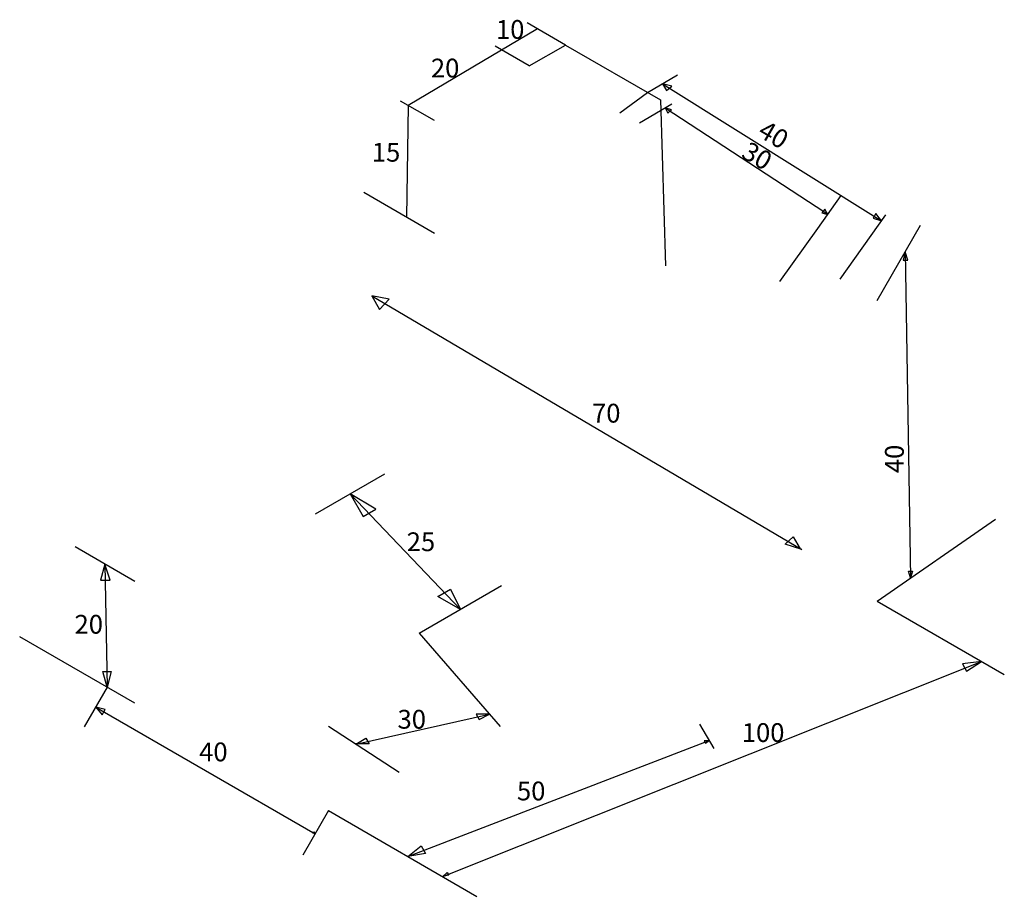
# Model space of a CAD drawing. Units: inches. Extents: x 17467 to 446717, y 8017 to 206428.
# Tile 1 of 2: x 17467 to 17598, y 8017 to 8134. Entities that reach past the tile are written whole.
import ezdxf

# ---------------------------------------------------------------- set-up
doc = ezdxf.new("R2010")
doc.units = ezdxf.units.IN
doc.layers.add('M-DIMS', color=2, linetype='Continuous', lineweight=25)
doc.layers.add('M-TEXT', color=7, linetype='Continuous', lineweight=25)
doc.styles.get("Standard").update_dxf_attribs({"font": 'arial.ttf'})

msp = doc.modelspace()

# ---------------------------------------------------------------- linework, layer by layer
at = {"layer": 'M-DIMS'}
for p, q in [((17539.99, 8130.15), (17534.91, 8133.09)), ((17536.29, 8132.29), (17519.07, 8122.12)), ((17535.19, 8127.38), (17539.99, 8130.15)), ((17539.99, 8130.15), (17552.65, 8122.84)), ((17535.19, 8127.38), (17530.64, 8130.01)), ((17550.91, 8123.85), (17554.91, 8126.16)), ((17552.91, 8125), (17582.07, 8106.74)), ((17552.91, 8125), (17553.45, 8124.08)), ((17554.14, 8124.69), (17552.91, 8125)), ((17547.26, 8121.13), (17550.91, 8123.85)), ((17553.45, 8124.08), (17554.14, 8124.69)), ((17522.57, 8120.09), (17518.07, 8122.69)), ((17549.84, 8119.79), (17554.18, 8122.3)), ((17552.65, 8122.84), (17553.33, 8100.75)), ((17519.07, 8122.12), (17518.87, 8107.23)), ((17553.26, 8121.77), (17574.5, 8107.89)), ((17553.26, 8121.77), (17553.65, 8121.09)), ((17554.12, 8121.53), (17553.26, 8121.77)), ((17553.65, 8121.09), (17554.12, 8121.53)), ((17522.57, 8105.09), (17513.16, 8110.53)), ((17573.57, 8105.75), (17576.68, 8110.11)), ((17574.5, 8108.29), (17574.11, 8107.83)), ((17574.9, 8107.6), (17574.5, 8108.29)), ((17574.5, 8107.89), (17574.9, 8107.6)), ((17574.11, 8107.83), (17574.9, 8107.6)), ((17576.57, 8098.99), (17582.64, 8107.54)), ((17581.31, 8107.72), (17580.97, 8107.12)), ((17580.97, 8107.12), (17582.07, 8106.74)), ((17582.07, 8106.74), (17581.31, 8107.72)), ((17568.52, 8098.66), (17573.57, 8105.75)), ((17581.47, 8096.15), (17587.26, 8106.17)), ((17585.21, 8102.63), (17584.94, 8101.54)), ((17585.21, 8102.63), (17585.94, 8059.25)), ((17585.57, 8101.54), (17585.21, 8102.63)), ((17584.94, 8101.54), (17585.57, 8101.54)), ((17514.25, 8096.76), (17571.46, 8063.03)), ((17514.25, 8096.76), (17515.28, 8094.97)), ((17516.55, 8096.33), (17514.25, 8096.76)), ((17515.28, 8094.97), (17516.55, 8096.33)), ((17506.76, 8067.78), (17515.97, 8073.1)), ((17511.36, 8070.44), (17526.02, 8055.05)), ((17511.36, 8070.44), (17513.1, 8067.43)), ((17514.77, 8068.4), (17511.36, 8070.44)), ((17513.1, 8067.43), (17514.77, 8068.4)), ((17581.47, 8056.15), (17597.22, 8067.06)), ((17569.25, 8063.73), (17570.29, 8064.72)), ((17570.29, 8064.72), (17571.22, 8063.11)), ((17482.72, 8058.76), (17474.75, 8063.36)), ((17571.46, 8063.03), (17569.25, 8063.73)), ((17478.73, 8061.06), (17478.12, 8058.96)), ((17478.73, 8061.06), (17479.02, 8044.7)), ((17479.4, 8058.96), (17478.73, 8061.06)), ((17585.94, 8059.25), (17585.67, 8060.14)), ((17585.67, 8060.14), (17586.19, 8060.14)), ((17586.19, 8060.14), (17585.94, 8059.25)), ((17478.12, 8058.96), (17479.4, 8058.96)), ((17520.55, 8051.9), (17531.49, 8058.21)), ((17523.04, 8056.78), (17524.7, 8057.74)), ((17526.02, 8055.05), (17523.04, 8056.78)), ((17524.7, 8057.74), (17526.02, 8055.05)), ((17581.47, 8056.15), (17598.4, 8046.38)), ((17520.55, 8051.9), (17531.32, 8039.48)), ((17482.72, 8042.57), (17467.38, 8051.42)), ((17523.67, 8019.51), (17595.35, 8048.14)), ((17595.35, 8048.14), (17592.82, 8047.81)), ((17592.82, 8047.81), (17593.37, 8046.85)), ((17593.37, 8046.85), (17595.35, 8048.14)), ((17479.02, 8044.7), (17475.97, 8039.41)), ((17477.5, 8042.05), (17506.7, 8025.2)), ((17477.5, 8042.05), (17478.34, 8041.04)), ((17478.74, 8041.72), (17477.5, 8042.05)), ((17478.34, 8041.04), (17478.74, 8041.72)), ((17512.13, 8037.13), (17529.89, 8041.12)), ((17529.89, 8041.12), (17528.12, 8041.12)), ((17528.12, 8041.12), (17528.54, 8040.41)), ((17528.54, 8040.41), (17529.89, 8041.12)), ((17557.86, 8039.8), (17559.73, 8036.55)), ((17508.48, 8039.51), (17517.87, 8033.38)), ((17513.88, 8037.18), (17512.06, 8037.18)), ((17512.13, 8037.13), (17513.46, 8037.9)), ((17513.46, 8037.9), (17513.88, 8037.18)), ((17519.02, 8022.19), (17559.13, 8037.6)), ((17559.13, 8037.6), (17558.47, 8037.55)), ((17558.47, 8037.55), (17558.66, 8037.23)), ((17558.66, 8037.23), (17559.13, 8037.6)), ((17508.48, 8028.28), (17505.05, 8022.35)), ((17508.48, 8028.28), (17528.23, 8016.87)), ((17506.4, 8025.28), (17506.5, 8025.45)), ((17506.5, 8025.45), (17506.7, 8025.2)), ((17506.7, 8025.2), (17506.4, 8025.28)), ((17519.02, 8022.19), (17520.8, 8023.59)), ((17520.8, 8023.59), (17521.4, 8022.55)), ((17521.4, 8022.55), (17519.02, 8022.19)), ((17523.67, 8019.51), (17524.28, 8020.05)), ((17524.28, 8020.05), (17524.49, 8019.68)), ((17524.49, 8019.68), (17523.67, 8019.51))]:
    msp.add_line(p, q, dxfattribs=at)
msp.add_lwpolyline([(17479.02, 8044.7), (17478.44, 8046.81), (17479.57, 8046.81), (17479.02, 8044.7)], dxfattribs=at)

# ---------------------------------------------------------------- texts
at = {"layer": 'M-TEXT', "char_height": 2.5, "attachment_point": 1}
for s, width, insert in [('10', 0.8845, (17530.76, 8133.47)), ('20', 2.0811, (17522.1, 8128.33)), ('15', 2.1713, (17514.24, 8117.13)), ('70', 10.8506, (17543.54, 8082.41)), ('25', 8.2046, (17518.88, 8065.3)), ('20', 1.6664, (17474.68, 8054.32)), ('30', 3.0478, (17517.66, 8041.68)), ('100', 3.9392, (17563.47, 8039.91)), ('40', 4.6882, (17491.26, 8037.34)), ('50', 6.5149, (17533.55, 8032.14))]:
    msp.add_mtext_dynamic_manual_height_columns(s, width=width, gutter_width=12.5, heights=[0], dxfattribs=dict(at, insert=insert))
for s, width, insert, rotation in [('40', 2.5458, (17566.69, 8120.25), 330), ('30', 2.036, (17564.5, 8117.42), 330), ('40', 1.4122, (17582.53, 8073.18), 90)]:
    msp.add_mtext_dynamic_manual_height_columns(s, width=width, gutter_width=12.5, heights=[0], dxfattribs=dict(at, insert=insert, rotation=rotation))

doc.saveas('drawing.dxf')
